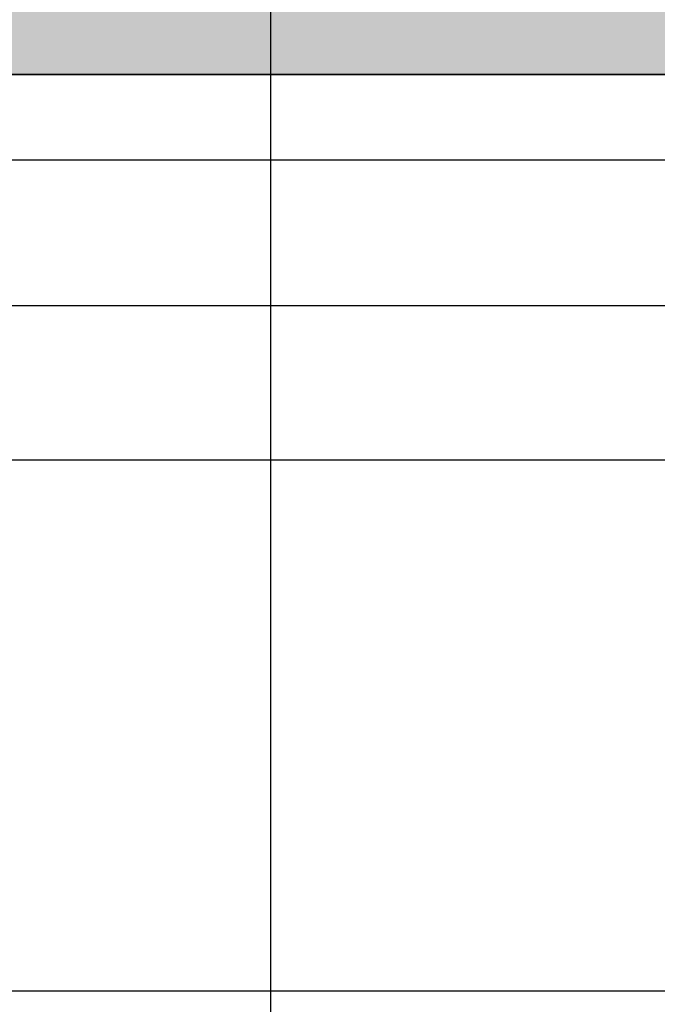
# Model space of a CAD drawing. Units: inches. Extents: x 2696 to 3240, y 1564 to 2310.
# Tile 22 of 76: x 2827 to 2864, y 1852 to 1910. Entities that reach past the tile are written whole.
import ezdxf

# ---------------------------------------------------------------- set-up
doc = ezdxf.new("R2010")
doc.units = ezdxf.units.IN
for name, color, linetype, lineweight in [('A-ANNO-DIMS', 3, 'Continuous', 18), ('A-WALL', 7, 'Continuous', 35), ('A-WALL-PATT', 9, 'Continuous', 13)]:
    doc.layers.add(name, color=color, linetype=linetype, lineweight=lineweight)
doc.styles.add('TIMES NEW', font='times.ttf')
doc.dimstyles.new('Siddhuu', dxfattribs={"dimtxt": 6, "dimasz": 2.5, "dimexe": 1.25, "dimexo": 0.625, "dimtad": 1, "dimdec": 1, "dimlunit": 4, "dimtxsty": 'TIMES NEW', "dimcen": 2.5, "dimclrd": 256, "dimclre": 1, "dimclrt": 7, "dimadec": 0, "dimazin": 0, "dimtfac": 1, "dimtdec": 1, "dimtmove": 0, "dimatfit": 3, "dimfxl": 1, "dimtolj": 1, "dimlwd": -1, "dimarcsym": 0})

# ---------------------------------------------------------------- blocks, each defined once
blk = doc.blocks.new('*D55')
at = {"layer": 'A-ANNO-DIMS', "color": 1, "lineweight": -2, "transparency": 16777216}
for p, q in [((3189.986, 1980.201), (2709.361, 1980.201)), ((3189.986, 1893.201), (2709.361, 1893.201))]:
    blk.add_line(p, q, dxfattribs=at)
at = {"layer": 'A-ANNO-DIMS', "transparency": 16777216}
blk.add_line((2710.611, 1895.701), (2710.611, 1977.701), dxfattribs=at)
for points in [[(2710.195, 1977.701), (2711.028, 1977.701), (2710.611, 1980.201)], [(2710.195, 1895.701), (2711.028, 1895.701), (2710.611, 1893.201)]]:
    blk.add_solid(points, dxfattribs=at)
at = {"layer": 'Defpoints', "color": 0, "transparency": 16777216}
for p in [(2710.611, 1980.201), (3190.611, 1980.201), (3190.611, 1893.201)]:
    blk.add_point(p, dxfattribs=at)
at = {"layer": 'A-ANNO-DIMS', "color": 7, "transparency": 16777216, "insert": (2706.926, 1936.701), "char_height": 6, "attachment_point": 5, "rotation": 90, "style": 'TIMES NEW'}
blk.add_mtext('\\A1;7\'-3"', dxfattribs=at)
blk = doc.blocks.new('*D57')
at = {"layer": 'A-ANNO-DIMS', "color": 1, "lineweight": -2, "transparency": 16777216}
for p, q in [((2754.611, 2018.576), (2754.611, 1568.951)), ((2956.709, 2018.576), (2956.709, 1568.951))]:
    blk.add_line(p, q, dxfattribs=at)
at = {"layer": 'A-ANNO-DIMS', "transparency": 16777216}
blk.add_line((2757.111, 1570.201), (2954.209, 1570.201), dxfattribs=at)
for points in [[(2757.111, 1570.618), (2757.111, 1569.784), (2754.611, 1570.201)], [(2954.209, 1570.618), (2954.209, 1569.784), (2956.709, 1570.201)]]:
    blk.add_solid(points, dxfattribs=at)
at = {"layer": 'Defpoints', "color": 0, "transparency": 16777216}
for p in [(2754.611, 2019.201), (2956.709, 2019.201), (2956.709, 1570.201)]:
    blk.add_point(p, dxfattribs=at)
at = {"layer": 'A-ANNO-DIMS', "color": 7, "transparency": 16777216, "insert": (2855.66, 1573.878), "char_height": 6, "attachment_point": 5, "style": 'TIMES NEW'}
blk.add_mtext('\\A1;16\'-10"', dxfattribs=at)
blk = doc.blocks.new('*D69')
at = {"layer": 'A-ANNO-DIMS', "color": 1, "lineweight": -2, "transparency": 16777216}
for p, q in [((2841.889, 2261.576), (2841.889, 1568.951)), ((2905.91, 2261.576), (2905.91, 1568.951))]:
    blk.add_line(p, q, dxfattribs=at)
at = {"layer": 'A-ANNO-DIMS', "transparency": 16777216}
blk.add_line((2844.389, 1570.201), (2903.41, 1570.201), dxfattribs=at)
for points in [[(2844.389, 1570.618), (2844.389, 1569.784), (2841.889, 1570.201)], [(2903.41, 1570.618), (2903.41, 1569.784), (2905.91, 1570.201)]]:
    blk.add_solid(points, dxfattribs=at)
at = {"layer": 'Defpoints', "color": 0, "transparency": 16777216}
for p in [(2841.889, 2262.201), (2905.91, 2262.201), (2905.91, 1570.201)]:
    blk.add_point(p, dxfattribs=at)
at = {"layer": 'A-ANNO-DIMS', "color": 7, "transparency": 16777216, "insert": (2873.9, 1573.878), "char_height": 6, "attachment_point": 5, "style": 'TIMES NEW'}
blk.add_mtext('\\A1;5\'-4"', dxfattribs=at)
blk = doc.blocks.new('*D78')
at = {"layer": 'A-ANNO-DIMS', "transparency": 16777216}
for p, q in [((2710.611, 1901.701), (2710.611, 1935.101)), ((2710.611, 1895.701), (2710.611, 1899.201))]:
    blk.add_line(p, q, dxfattribs=at)
at = {"layer": 'A-ANNO-DIMS', "color": 1, "lineweight": -2, "transparency": 16777216}
for p, q in [((3189.986, 1901.701), (2709.361, 1901.701)), ((3189.986, 1893.201), (2709.361, 1893.201))]:
    blk.add_line(p, q, dxfattribs=at)
at = {"layer": 'A-ANNO-DIMS', "transparency": 16777216}
for points in [[(2710.195, 1899.201), (2711.028, 1899.201), (2710.611, 1901.701)], [(2710.195, 1895.701), (2711.028, 1895.701), (2710.611, 1893.201)]]:
    blk.add_solid(points, dxfattribs=at)
at = {"layer": 'Defpoints', "color": 0, "transparency": 16777216}
for p in [(2710.611, 1901.701), (3190.611, 1901.701), (3190.611, 1893.201)]:
    blk.add_point(p, dxfattribs=at)
at = {"layer": 'A-ANNO-DIMS', "color": 7, "transparency": 16777216, "insert": (2706.85, 1919.651), "char_height": 6, "attachment_point": 5, "rotation": 90, "style": 'TIMES NEW'}
blk.add_mtext('\\A1;0\'-8 1/2"', dxfattribs=at)
blk = doc.blocks.new('*D79')
at = {"layer": 'A-ANNO-DIMS', "color": 1, "lineweight": -2, "transparency": 16777216}
for p, q in [((3189.986, 1884.201), (2709.361, 1884.201)), ((3189.986, 1853.201), (2709.361, 1853.201))]:
    blk.add_line(p, q, dxfattribs=at)
at = {"layer": 'A-ANNO-DIMS', "transparency": 16777216}
blk.add_line((2710.611, 1881.701), (2710.611, 1855.701), dxfattribs=at)
for points in [[(2710.195, 1881.701), (2711.028, 1881.701), (2710.611, 1884.201)], [(2710.195, 1855.701), (2711.028, 1855.701), (2710.611, 1853.201)]]:
    blk.add_solid(points, dxfattribs=at)
at = {"layer": 'Defpoints', "color": 0, "transparency": 16777216}
for p in [(3190.611, 1884.201), (2710.611, 1853.201), (3190.611, 1853.201)]:
    blk.add_point(p, dxfattribs=at)
at = {"layer": 'A-ANNO-DIMS', "color": 7, "transparency": 16777216, "insert": (2706.926, 1868.701), "char_height": 6, "attachment_point": 5, "rotation": 90, "style": 'TIMES NEW'}
blk.add_mtext('\\A1;2\'-7"', dxfattribs=at)

msp = doc.modelspace()

# ---------------------------------------------------------------- hatches: boundary and pattern name
at = {"layer": 'A-WALL-PATT', "transparency": 33554556}
h = msp.add_hatch(color=256, dxfattribs=at)
h.dxf.hatch_style = 1
h.paths.add_polyline_path([(2879.111, 2253.201), (2905.91, 2253.201), (2905.91, 2262.201), (2841.889, 2262.201), (2841.889, 2253.201), (2870.111, 2253.201), (2870.111, 2176.601), (2965.709, 2176.601), (2965.709, 2206.701), (2973.583, 2206.701), (2973.583, 2215.701), (2965.709, 2215.701), (2965.709, 2262.201), (2929.91, 2262.201), (2929.91, 2253.201), (2956.709, 2253.201), (2956.709, 2185.601), (2879.111, 2185.601)])
h.paths.add_polyline_path([(2782.834, 2262.201), (2745.611, 2262.201), (2745.611, 2228.729), (2754.611, 2228.729), (2754.611, 2253.201), (2782.834, 2253.201)])
h.paths.add_polyline_path([(2754.611, 2136.201), (2965.709, 2136.201), (2965.709, 2145.201), (2879.111, 2145.201), (2879.111, 2147.074), (2877.34, 2147.074), (2870.111, 2147.074), (2870.111, 2145.201), (2754.611, 2145.201), (2754.611, 2169.674), (2745.611, 2169.674), (2745.611, 2000.201), (2754.611, 2000.201), (2754.611, 2019.201), (2849.083, 2019.201), (2849.083, 2023.701), (2841.209, 2023.701), (2841.209, 2051.827), (2836.709, 2051.827), (2836.709, 2023.701), (2754.611, 2023.701), (2754.611, 2091.201), (2836.709, 2091.201), (2836.709, 2087.827), (2841.209, 2087.827), (2841.209, 2095.701), (2754.611, 2095.701)])
h.paths.add_polyline_path([(2965.709, 2136.201), (2956.709, 2136.201), (2956.709, 2023.701), (2885.083, 2023.701), (2885.083, 2019.201), (2956.709, 2019.201), (2956.709, 1950.575), (2965.709, 1950.575), (2965.709, 1980.201), (2973.583, 1980.201), (2973.583, 1989.201), (2965.709, 1989.201)])
h.paths.add_polyline_path([(2754.611, 1906.701), (2880.209, 1906.701), (2884.709, 1906.701), (2956.709, 1906.701), (2956.709, 1792.701), (2944.709, 1792.701), (2944.709, 1783.701), (2956.709, 1783.701), (2956.709, 1740.201), (2884.709, 1740.201), (2884.709, 1783.701), (2896.709, 1783.701), (2896.709, 1792.701), (2884.709, 1792.701), (2884.709, 1846.701), (2880.209, 1846.701), (2880.209, 1740.201), (2754.611, 1740.201), (2754.611, 1777.201), (2745.611, 1777.201), (2745.611, 1692.701), (2754.611, 1692.701), (2754.611, 1731.201), (2956.709, 1731.201), (2956.709, 1723.327), (2965.709, 1723.327), (2965.709, 1884.201), (2973.583, 1884.201), (2973.583, 1893.201), (2965.709, 1893.201), (2965.709, 1914.575), (2956.709, 1914.575), (2956.709, 1911.201), (2754.611, 1911.201), (2754.611, 1930.201), (2745.611, 1930.201), (2745.611, 1817.201), (2754.611, 1817.201), (2754.611, 1854.201), (2826.611, 1854.201), (2826.611, 1868.827), (2822.111, 1868.827), (2822.111, 1858.701), (2754.611, 1858.701)])
h.paths.add_polyline_path([(2965.709, 1656.201), (3008.237, 1656.201), (3008.237, 1665.201), (2965.709, 1665.201), (2965.709, 1693.327), (2956.709, 1693.327), (2956.709, 1686.201), (2934.583, 1686.201), (2934.583, 1681.701), (2956.709, 1681.701), (2956.709, 1614.201), (2896.709, 1614.201), (2896.709, 1681.701), (2904.583, 1681.701), (2904.583, 1686.201), (2892.209, 1686.201), (2892.209, 1614.201), (2858.41, 1614.201), (2858.41, 1605.201), (2965.709, 1605.201)])
h.paths.add_polyline_path([(2788.41, 1614.201), (2754.611, 1614.201), (2754.611, 1652.701), (2745.611, 1652.701), (2745.611, 1605.201), (2788.41, 1605.201)])
h.paths.add_polyline_path([(3199.611, 1633.048), (3190.611, 1633.048), (3190.611, 1614.201), (3082.611, 1614.201), (3082.611, 1665.201), (3070.237, 1665.201), (3070.237, 1656.201), (3078.111, 1656.201), (3078.111, 1605.201), (3199.611, 1605.201)])
h.paths.add_polyline_path([(3199.611, 1702.048), (3190.611, 1702.048), (3190.611, 1699.701), (3106.611, 1699.701), (3106.611, 1747.701), (3190.611, 1747.701), (3190.611, 1752.201), (3082.611, 1752.201), (3082.611, 1760.075), (3078.111, 1760.075), (3078.111, 1747.701), (3102.111, 1747.701), (3102.111, 1699.701), (3078.111, 1699.701), (3078.111, 1695.201), (3190.611, 1695.201), (3190.611, 1676.355), (3199.611, 1676.355)])
h.paths.add_polyline_path([(3199.611, 1783.201), (3190.611, 1783.201), (3190.611, 1745.355), (3199.611, 1745.355)])
h.paths.add_polyline_path([(3082.611, 1884.201), (3190.611, 1884.201), (3190.611, 1853.201), (3199.611, 1853.201), (3199.611, 1901.701), (3190.611, 1901.701), (3190.611, 1893.201), (3005.583, 1893.201), (3005.583, 1891.281), (3005.583, 1884.201), (3078.111, 1884.201), (3078.111, 1792.075), (3082.611, 1792.075)])
h.paths.add_polyline_path([(3199.611, 1994.701), (3190.611, 1994.701), (3190.611, 1989.201), (3073.709, 1989.201), (3073.709, 2034.201), (3069.209, 2034.201), (3069.209, 1989.201), (3005.583, 1989.201), (3005.583, 1980.201), (3190.611, 1980.201), (3190.611, 1971.701), (3199.611, 1971.701)])
h.paths.add_polyline_path([(3199.611, 2155.201), (3190.611, 2155.201), (3190.611, 2064.701), (3199.611, 2064.701)])
h.paths.add_polyline_path([(3190.611, 2074.701), (3106.611, 2074.701), (3106.611, 2122.701), (3190.611, 2122.701), (3190.611, 2127.201), (3082.709, 2127.201), (3082.709, 2135.075), (3073.709, 2135.075), (3073.709, 2122.701), (3102.111, 2122.701), (3102.111, 2074.701), (3069.209, 2074.701), (3069.209, 2070.201), (3190.611, 2070.201)])
h.paths.add_polyline_path([(3082.709, 2253.201), (3190.611, 2253.201), (3190.611, 2225.201), (3199.611, 2225.201), (3199.611, 2262.201), (3073.709, 2262.201), (3073.709, 2215.701), (3035.583, 2215.701), (3035.583, 2206.701), (3073.709, 2206.701), (3073.709, 2171.075), (3082.709, 2171.075)])

# ---------------------------------------------------------------- linework, layer by layer
at = {"layer": 'A-WALL'}
msp.add_line((2754.611, 1906.701), (2880.209, 1906.701), dxfattribs=at)

# ---------------------------------------------------------------- dimensions: what is measured, and where the dimension line sits
at = {"layer": 'A-ANNO-DIMS'}
for base, p1, p2, picture, middle in [((2905.91, 1570.201), (2841.889, 2262.201), (2905.91, 2262.201), '*D69', (2873.9, 1573.878)), ((2956.709, 1570.201), (2754.611, 2019.201), (2956.709, 2019.201), '*D57', (2855.66, 1573.878))]:
    dim = msp.add_linear_dim(base=base, p1=p1, p2=p2, dimstyle='Siddhuu', override={"dimdec": 1, "dimlfac": 1, "dimrnd": 0, "dimzin": 1, "dimdsep": 46, "dimlunit": 4, "dimfrac": 2}, dxfattribs=at)
    dim.commit()
    dim.dimension.update_dxf_attribs({"geometry": picture, "text_midpoint": middle})
for base, p1, p2, picture, middle in [((2710.611, 1980.201), (3190.611, 1893.201), (3190.611, 1980.201), '*D55', (2706.926, 1936.701)), ((2710.611, 1901.701), (3190.611, 1893.201), (3190.611, 1901.701), '*D78', (2706.85, 1919.651)), ((2710.611, 1853.201), (3190.611, 1884.201), (3190.611, 1853.201), '*D79', (2706.926, 1868.701))]:
    dim = msp.add_linear_dim(base=base, p1=p1, p2=p2, angle=90, dimstyle='Siddhuu', override={"dimdec": 1, "dimlfac": 1, "dimrnd": 0, "dimzin": 1, "dimdsep": 46, "dimlunit": 4, "dimfrac": 2}, dxfattribs=at)
    dim.commit()
    dim.dimension.update_dxf_attribs({"geometry": picture, "text_midpoint": middle})

doc.saveas('drawing.dxf')
